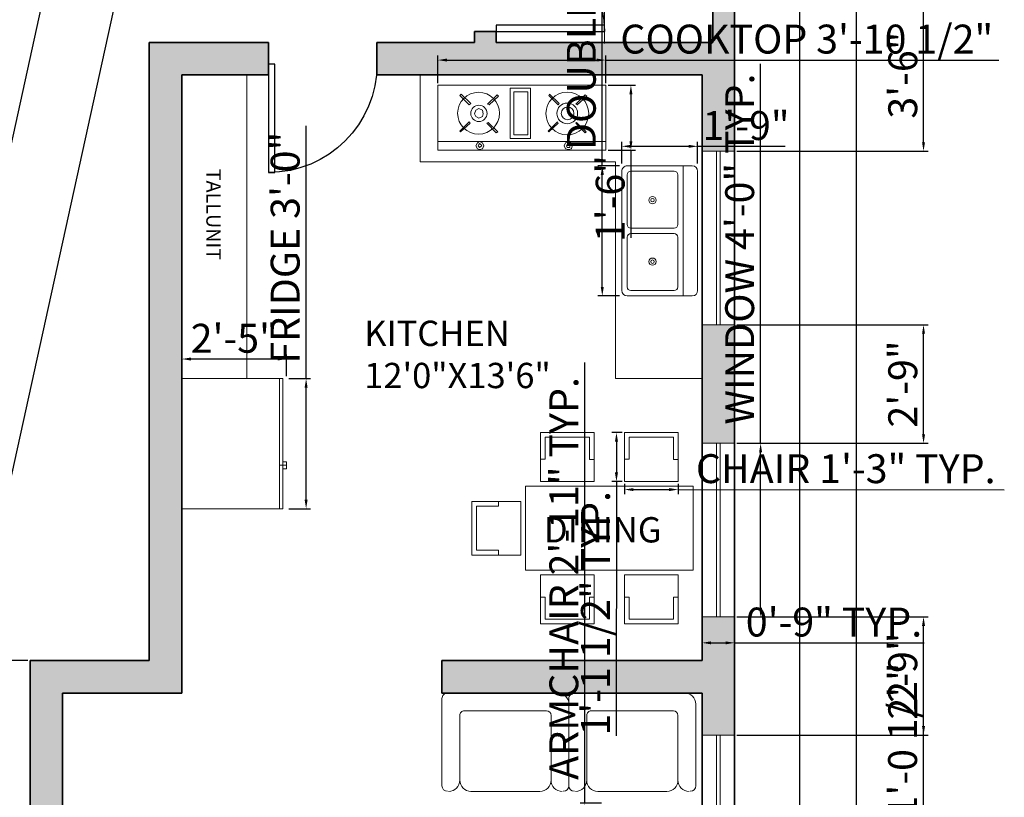
# Model space of a CAD drawing. Units: inches. Extents: x 2642 to 4124, y 1227 to 1973.
# Tile 5 of 7: x 3483 to 3756, y 1645 to 1860. Entities that reach past the tile are written whole.
import ezdxf

# ---------------------------------------------------------------- set-up
doc = ezdxf.new("R2010")
doc.units = ezdxf.units.IN
for name, color, linetype, lineweight in [('A-ANNO-DIMS', 2, 'Continuous', 18), ('A-ANNO-TEXT', 7, 'Continuous', 18), ('A-AREA-IDEN', 7, 'Continuous', 18), ('A-DOOR', 3, 'Continuous', 25), ('A-EQPM', 8, 'Continuous', 18), ('A-FLOR-CASE', 8, 'Continuous', 18), ('A-WALL', 7, 'Continuous', 35), ('A-WALL-PATT', 7, 'Continuous', 13), ('C-PROP', 7, 'Continuous', 25), ('furn', 165, 'Continuous', 18), ('window', 4, 'Continuous', 18), ('Сантехника', 9, 'Continuous', 18)]:
    doc.layers.add(name, color=color, linetype=linetype, lineweight=lineweight)
doc.styles.get("Standard").update_dxf_attribs({"font": 'arial.ttf'})
doc.dimstyles.new('ISO-25', dxfattribs={"dimtxt": 8, "dimasz": 2.5, "dimexe": 1.25, "dimexo": 0.625, "dimtad": 1, "dimdec": 0, "dimlunit": 3, "dimtxsty": 'Standard', "dimcen": 2.5, "dimadec": 0, "dimazin": 0, "dimtfac": 1, "dimtdec": 0, "dimtmove": 0, "dimatfit": 3, "dimfxl": 1, "dimarcsym": 0})

# ---------------------------------------------------------------- blocks, each defined once
blk = doc.blocks.new('*D2')
at = {"layer": 'A-ANNO-DIMS', "color": 0, "lineweight": -2, "transparency": 16777216}
for p, q in [((3699.85, 1907.78), (3716.14, 1907.78)), ((3714.89, 1905.28), (3714.89, 1310.28)), ((3699.85, 1307.78), (3716.14, 1307.78))]:
    blk.add_line(p, q, dxfattribs=at)
at = {"layer": 'A-ANNO-DIMS', "color": 0, "transparency": 16777216}
for points in [[(3714.47, 1905.28), (3715.3, 1905.28), (3714.89, 1907.78)], [(3714.47, 1310.28), (3715.3, 1310.28), (3714.89, 1307.78)]]:
    blk.add_solid(points, dxfattribs=at)
at = {"layer": 'Defpoints', "color": 0, "transparency": 16777216}
for p in [(3699.22, 1907.78), (3699.22, 1307.78), (3714.89, 1307.78)]:
    blk.add_point(p, dxfattribs=at)
at = {"layer": 'A-ANNO-DIMS', "color": 0, "transparency": 16777216, "insert": (3710.18, 1607.78), "char_height": 8, "attachment_point": 5, "rotation": 90}
blk.add_mtext("50'", dxfattribs=at)
blk = doc.blocks.new('*D4')
at = {"layer": 'A-ANNO-DIMS', "color": 0, "lineweight": -2, "transparency": 16777216}
for p, q in [((3518.61, 1907.92), (3498.8, 1912.28)), ((3368.56, 1314.45), (3499.49, 1909.57)), ((3386.61, 1307.92), (3366.8, 1312.28))]:
    blk.add_line(p, q, dxfattribs=at)
at = {"layer": 'A-ANNO-DIMS', "color": 0, "transparency": 16777216}
for points in [[(3499.08, 1909.65), (3499.89, 1909.48), (3500.02, 1912.01)], [(3368.15, 1314.54), (3368.97, 1314.36), (3368.02, 1312.01)]]:
    blk.add_solid(points, dxfattribs=at)
at = {"layer": 'Defpoints', "color": 0, "transparency": 16777216}
for p in [(3500.02, 1912.01), (3519.22, 1907.78), (3387.22, 1307.78)]:
    blk.add_point(p, dxfattribs=at)
at = {"layer": 'A-ANNO-DIMS', "color": 0, "transparency": 16777216, "insert": (3429.42, 1613.02), "char_height": 8, "attachment_point": 5, "rotation": 77.5926}
blk.add_mtext('51\'-2"', dxfattribs=at)
blk = doc.blocks.new('*U11')
for p, q in [((0, 0), (0, -6)), ((30, 0), (30, -6))]:
    blk.add_line(p, q)
blk.add_lwpolyline([(0, 0), (0, 30), (1.75, 30), (1.75, 0)], close=True)
blk.add_arc((0, 0), 30, 0, 90)
blk = doc.blocks.new('sofa-27')
at = {"color": 0, "linetype": 'ByBlock'}
for p, q in [((-0.0591, 0.0591), (-0.0591, 0.4902)), ((0.0945, 0.5198), (0.459, 0.5198)), ((0.6125, 0.0295), (0.6125, 0.4902)), ((0.0354, 0.1181), (0.0354, 0.4607)), ((0.518, 0.1181), (0.518, 0.4607)), ((0.4944, 0.0945), (0.0591, 0.0945)), ((0.583, 0), (0, 0))]:
    blk.add_line(p, q, dxfattribs=at)
for centre, radius, start, end in [((-0.0295, 0.4902), 0.0295, 90, 180), ((-0.0236, 0.4607), 0.0591, 360, 90), ((0.0945, 0.4607), 0.0591, 90, 180), ((0.459, 0.4607), 0.0591, 0, 90), ((0.5771, 0.4607), 0.0591, 90, 180), ((0.583, 0.4902), 0.0295, 0, 90), ((0.0591, 0.1181), 0.0236, 180, 270), ((0.4944, 0.1181), 0.0236, 270, 0), ((0, 0.0591), 0.0591, 180, 270), ((0.583, 0.0295), 0.0295, 270, 0)]:
    blk.add_arc(centre, radius, start, end, dxfattribs=at)
blk = doc.blocks.new('gas 1')
for points in [[(35.93, -1.87), (35.93, 0), (0, 0), (0, -1.87)], [(8.12, -0.94), (8.44, -1.56), (8.91, -1.87), (9.53, -1.56), (9.84, -0.94), (9.53, -0.31), (8.91, -0.16), (8.44, -0.31)], [(8.59, -0.94), (8.75, -1.25), (8.91, -1.41), (9.22, -1.25), (9.37, -0.94), (9.22, -0.78), (8.91, -0.62), (8.75, -0.78)], [(27.03, -0.94), (27.34, -1.56), (27.97, -1.87), (28.59, -1.56), (28.75, -0.94), (28.59, -0.31), (27.97, -0.16), (27.34, -0.31)], [(27.5, -0.94), (27.65, -1.25), (27.97, -1.41), (28.28, -1.25), (28.28, -0.94), (28.28, -0.62), (27.97, -0.62), (27.65, -0.62)], [(4.84, -3.91), (4.69, -4.06), (6.72, -6.09), (6.87, -5.78)], [(12.81, -3.91), (12.5, -3.75), (10.47, -5.78), (10.78, -5.94)], [(19.84, -13.28), (15.47, -13.28), (15.47, -2.5), (19.84, -2.5)], [(19.22, -12.5), (16.25, -12.5), (16.25, -3.28), (19.22, -3.28)], [(23.75, -3.91), (23.59, -4.06), (25.62, -6.09), (25.78, -5.78)], [(31.71, -3.91), (31.56, -3.75), (29.53, -5.78), (29.68, -5.94)], [(7.81, -7.81), (8.12, -8.59), (8.75, -8.91), (9.53, -8.59), (9.69, -7.81), (9.53, -7.19), (8.75, -6.87), (8.12, -7.19)], [(7.03, -10), (6.72, -9.69), (4.69, -11.72), (5, -12.03)], [(12.97, -11.56), (10.94, -9.69), (10.62, -9.84), (12.65, -11.87)], [(23.75, -11.72), (23.9, -12.03), (25.93, -10), (25.78, -9.69)], [(31.87, -11.56), (29.84, -9.69), (29.53, -9.84), (31.56, -11.87)]]:
    blk.add_lwpolyline(points, close=True)
blk.add_lwpolyline([(35.93, -1.87), (35.93, -13.9), (0, -13.9), (0, -1.87)])
for centre, radius in [((8.7, -7.92), 4.48), ((27.7, -7.86), 4.58), ((8.77, -7.89), 1.74), ((27.69, -7.89), 2.22), ((27.76, -7.89), 1.35)]:
    blk.add_circle(centre, radius)
blk = doc.blocks.new('Sink-double - 36 in top')
for p, q in [((-18, -4), (18, -4)), ((-0.75, -18.5), (-0.75, -6.5)), ((0.75, -6.5), (0.75, -18.5))]:
    blk.add_line(p, q)
for points in [[(-16.5, 0), (16.5, 0)], [(-18, -19.5), (-18, -1.5)], [(18, -1.5), (18, -19.5)], [(-16.5, -18.5), (-16.5, -6.5)], [(-15.5, -5.5), (-1.75, -5.5)], [(1.75, -5.5), (15.5, -5.5)], [(16.5, -6.5), (16.5, -18.5)], [(16.5, -21), (-16.5, -21)], [(-1.75, -19.5), (-15.5, -19.5)], [(15.5, -19.5), (1.75, -19.5)]]:
    blk.add_lwpolyline(points)
for centre, radius in [((-8.5, -12.5), 1), ((-8.5, -12.5), 0.5), ((8.5, -12.5), 1), ((8.5, -12.5), 0.5)]:
    blk.add_circle(centre, radius)
for centre, radius, start, end in [((-16.5, -1.5), 1.5, 90, 180), ((16.5, -1.5), 1.5, 0, 90), ((-15.5, -6.5), 1, 90, 180), ((-1.75, -6.5), 1, 0, 90), ((1.75, -6.5), 1, 90, 180), ((15.5, -6.5), 1, 0, 90), ((-15.5, -18.5), 1, 180, 270), ((-1.75, -18.5), 1, 270, 0), ((1.75, -18.5), 1, 180, 270), ((15.5, -18.5), 1, 270, 0), ((-16.5, -19.5), 1.5, 180, 270), ((16.5, -19.5), 1.5, 270, 0)]:
    blk.add_arc(centre, radius, start, end)
blk = doc.blocks.new('Refrigerator-2 door - 36 in top')
for p, q in [((0, -26.999999), (36, -26.999999)), ((12, -26.999999), (12, -28.999999)), ((11, -27.999999), (11, -28.999999)), ((11, -28.999999), (13, -28.999999)), ((13, -28.999999), (13, -27.999999))]:
    blk.add_line(p, q)
blk.add_lwpolyline([(0, -27.999999), (0, 0), (36, 0), (36, -27.999999)], close=True)
blk = doc.blocks.new('CHAIR-DINING')
for p, q in [((0, 14.84), (13.57, 14.84)), ((0, 0), (0, 14.84)), ((7.42, 13.56), (7.42, 14.84)), ((13.57, 0), (13.57, 14.84)), ((1.28, 13.56), (7.42, 13.56)), ((1.28, 1.32), (1.28, 13.56)), ((0, 0), (13.57, 0)), ((7.42, 1.32), (1.28, 1.32)), ((7.42, 0), (7.42, 1.32))]:
    blk.add_line(p, q)
blk = doc.blocks.new('WIN-24IN')
for p, q in [((0, 24), (9, 24)), ((4, 24), (4, 0)), ((5, 24), (5, 0)), ((0, 0), (9, 0))]:
    blk.add_line(p, q)
blk = doc.blocks.new('WIN-48IN')
for p, q in [((9, 48), (0, 48)), ((4, 48), (4, 0)), ((5, 48), (5, 0)), ((9, 0), (0, 0))]:
    blk.add_line(p, q)
blk = doc.blocks.new('*D38')
at = {"layer": 'A-ANNO-DIMS', "color": 0, "lineweight": -2, "transparency": 16777216}
for p, q in [((3650.74, 1731.67), (3650.74, 1728.82)), ((3665.58, 1731.67), (3665.58, 1728.82)), ((3653.24, 1730.07), (3663.08, 1730.07)), ((3665.58, 1730.07), (3755.88, 1730.03))]:
    blk.add_line(p, q, dxfattribs=at)
at = {"layer": 'A-ANNO-DIMS', "color": 0, "transparency": 16777216}
for points in [[(3653.24, 1730.49), (3653.24, 1729.65), (3650.74, 1730.07)], [(3663.08, 1730.48), (3663.08, 1729.65), (3665.58, 1730.07)]]:
    blk.add_solid(points, dxfattribs=at)
at = {"layer": 'Defpoints', "color": 0, "transparency": 16777216}
for p in [(3650.74, 1732.3), (3665.58, 1732.29), (3665.58, 1730.07)]:
    blk.add_point(p, dxfattribs=at)
at = {"layer": 'A-ANNO-DIMS', "color": 0, "transparency": 16777216, "insert": (3711.98, 1734.81), "char_height": 8, "attachment_point": 5, "rotation": 359.979}
blk.add_mtext('CHAIR 1\'-3" TYP.', dxfattribs=at)
blk = doc.blocks.new('*D39')
at = {"layer": 'A-ANNO-DIMS', "color": 0, "lineweight": -2, "transparency": 16777216}
for p, q in [((3650.12, 1745.86), (3647.27, 1745.87)), ((3648.52, 1743.36), (3648.52, 1734.8)), ((3650.12, 1732.3), (3647.27, 1732.3)), ((3648.52, 1732.3), (3648.49, 1661.9))]:
    blk.add_line(p, q, dxfattribs=at)
at = {"layer": 'A-ANNO-DIMS', "color": 0, "transparency": 16777216}
for points in [[(3648.11, 1743.37), (3648.94, 1743.36), (3648.52, 1745.86)], [(3648.1, 1734.8), (3648.94, 1734.8), (3648.52, 1732.3)]]:
    blk.add_solid(points, dxfattribs=at)
at = {"layer": 'Defpoints', "color": 0, "transparency": 16777216}
for p in [(3650.75, 1745.86), (3648.52, 1732.3), (3650.74, 1732.3)]:
    blk.add_point(p, dxfattribs=at)
at = {"layer": 'A-ANNO-DIMS', "color": 0, "transparency": 16777216, "insert": (3643.74, 1695.85), "char_height": 8, "attachment_point": 5, "rotation": 89.979}
blk.add_mtext('1\'-1 1/2" TYP.', dxfattribs=at)
blk = doc.blocks.new('*D40')
at = {"layer": 'A-ANNO-DIMS', "color": 0, "lineweight": -2, "transparency": 16777216}
for p, q in [((3639.76, 1643.28), (3639.76, 1765.19)), ((3644.41, 1643.28), (3638.51, 1643.28)), ((3639.76, 1610.65), (3639.76, 1640.78)), ((3644.41, 1608.15), (3638.51, 1608.15))]:
    blk.add_line(p, q, dxfattribs=at)
at = {"layer": 'A-ANNO-DIMS', "color": 0, "transparency": 16777216}
for points in [[(3639.34, 1640.78), (3640.18, 1640.78), (3639.76, 1643.28)], [(3639.34, 1610.65), (3640.18, 1610.65), (3639.76, 1608.15)]]:
    blk.add_solid(points, dxfattribs=at)
at = {"layer": 'Defpoints', "color": 0, "transparency": 16777216}
for p in [(3639.76, 1643.28), (3645.03, 1643.28), (3645.03, 1608.15)]:
    blk.add_point(p, dxfattribs=at)
at = {"layer": 'A-ANNO-DIMS', "color": 0, "transparency": 16777216, "insert": (3635, 1705.48), "char_height": 8, "attachment_point": 5, "rotation": 90}
blk.add_mtext('ARMCHAIR 2\'-11" TYP.', dxfattribs=at)
blk = doc.blocks.new('*D44')
at = {"layer": 'A-ANNO-DIMS', "color": 0, "lineweight": -2, "transparency": 16777216}
for p, q in [((3688.42, 1742.87), (3688.42, 1847.85)), ((3681.85, 1742.87), (3689.67, 1742.87)), ((3688.42, 1697.37), (3688.42, 1740.37)), ((3681.85, 1694.87), (3689.67, 1694.87))]:
    blk.add_line(p, q, dxfattribs=at)
at = {"layer": 'A-ANNO-DIMS', "color": 0, "transparency": 16777216}
for points in [[(3688.01, 1740.37), (3688.84, 1740.37), (3688.42, 1742.87)], [(3688.01, 1697.37), (3688.84, 1697.37), (3688.42, 1694.87)]]:
    blk.add_solid(points, dxfattribs=at)
at = {"layer": 'Defpoints', "color": 0, "transparency": 16777216}
for p in [(3681.22, 1742.87), (3688.42, 1742.87), (3681.22, 1694.87)]:
    blk.add_point(p, dxfattribs=at)
at = {"layer": 'A-ANNO-DIMS', "color": 0, "transparency": 16777216, "insert": (3683.66, 1796.61), "char_height": 8, "attachment_point": 5, "rotation": 90}
blk.add_mtext('WINDOW 4\'-0" TYP.', dxfattribs=at)
blk = doc.blocks.new('*D45')
at = {"layer": 'A-ANNO-DIMS', "color": 0, "lineweight": -2, "transparency": 16777216}
for p, q in [((3672.22, 1694.24), (3672.22, 1686.42)), ((3681.22, 1694.24), (3681.22, 1686.42)), ((3674.72, 1687.67), (3678.72, 1687.67)), ((3681.22, 1687.67), (3733.74, 1687.67))]:
    blk.add_line(p, q, dxfattribs=at)
at = {"layer": 'A-ANNO-DIMS', "color": 0, "transparency": 16777216}
for points in [[(3674.72, 1688.08), (3674.72, 1687.25), (3672.22, 1687.67)], [(3678.72, 1688.08), (3678.72, 1687.25), (3681.22, 1687.67)]]:
    blk.add_solid(points, dxfattribs=at)
at = {"layer": 'Defpoints', "color": 0, "transparency": 16777216}
for p in [(3672.22, 1694.87), (3681.22, 1694.87), (3681.22, 1687.67)]:
    blk.add_point(p, dxfattribs=at)
at = {"layer": 'A-ANNO-DIMS', "color": 0, "transparency": 16777216, "insert": (3708.73, 1692.38), "char_height": 8, "attachment_point": 5}
blk.add_mtext('0\'-9" TYP.', dxfattribs=at)
blk = doc.blocks.new('*D58')
at = {"layer": 'A-ANNO-DIMS', "color": 0, "lineweight": -2, "transparency": 16777216}
for p, q in [((3599.11, 1842.55), (3599.11, 1850.14)), ((3601.61, 1848.89), (3643.06, 1848.89)), ((3645.56, 1842.55), (3645.56, 1850.14)), ((3645.56, 1848.89), (3754.33, 1848.89))]:
    blk.add_line(p, q, dxfattribs=at)
at = {"layer": 'A-ANNO-DIMS', "color": 0, "transparency": 16777216}
for points in [[(3601.61, 1849.31), (3601.61, 1848.48), (3599.11, 1848.89)], [(3643.06, 1849.31), (3643.06, 1848.48), (3645.56, 1848.89)]]:
    blk.add_solid(points, dxfattribs=at)
at = {"layer": 'Defpoints', "color": 0, "transparency": 16777216}
for p in [(3645.56, 1848.89), (3599.11, 1841.93), (3645.56, 1841.93)]:
    blk.add_point(p, dxfattribs=at)
at = {"layer": 'A-ANNO-DIMS', "color": 0, "transparency": 16777216, "insert": (3701.2, 1853.66), "char_height": 8, "attachment_point": 5}
blk.add_mtext('COOKTOP 3\'-10 1/2"', dxfattribs=at)
blk = doc.blocks.new('*D59')
at = {"layer": 'A-ANNO-DIMS', "color": 0, "lineweight": -2, "transparency": 16777216}
for p, q in [((3646.19, 1841.93), (3653.78, 1841.93)), ((3652.53, 1839.43), (3652.53, 1826.45)), ((3646.19, 1823.95), (3653.78, 1823.95)), ((3652.53, 1823.95), (3652.53, 1799.69))]:
    blk.add_line(p, q, dxfattribs=at)
at = {"layer": 'A-ANNO-DIMS', "color": 0, "transparency": 16777216}
for points in [[(3652.11, 1839.43), (3652.94, 1839.43), (3652.53, 1841.93)], [(3652.11, 1826.45), (3652.94, 1826.45), (3652.53, 1823.95)]]:
    blk.add_solid(points, dxfattribs=at)
at = {"layer": 'Defpoints', "color": 0, "transparency": 16777216}
for p in [(3645.56, 1841.93), (3645.56, 1823.95), (3652.53, 1823.95)]:
    blk.add_point(p, dxfattribs=at)
at = {"layer": 'A-ANNO-DIMS', "color": 0, "transparency": 16777216, "insert": (3647.82, 1810.57), "char_height": 8, "attachment_point": 5, "rotation": 90}
blk.add_mtext('1\'-6"', dxfattribs=at)
blk = doc.blocks.new('*D60')
at = {"layer": 'A-ANNO-DIMS', "color": 0, "lineweight": -2, "transparency": 16777216}
for p, q in [((3644.6, 1819.63), (3644.6, 1922.5)), ((3649.37, 1819.63), (3643.35, 1819.63)), ((3644.6, 1786.13), (3644.6, 1817.13)), ((3649.37, 1783.63), (3643.35, 1783.63))]:
    blk.add_line(p, q, dxfattribs=at)
at = {"layer": 'A-ANNO-DIMS', "color": 0, "transparency": 16777216}
for points in [[(3644.18, 1817.13), (3645.02, 1817.13), (3644.6, 1819.63)], [(3644.18, 1786.13), (3645.02, 1786.13), (3644.6, 1783.63)]]:
    blk.add_solid(points, dxfattribs=at)
at = {"layer": 'Defpoints', "color": 0, "transparency": 16777216}
for p in [(3644.6, 1819.63), (3650, 1819.63), (3650, 1783.63)]:
    blk.add_point(p, dxfattribs=at)
at = {"layer": 'A-ANNO-DIMS', "color": 0, "transparency": 16777216, "insert": (3639.83, 1872.32), "char_height": 8, "attachment_point": 5, "rotation": 90}
blk.add_mtext('DOUBLE SINK 3\'-0"', dxfattribs=at)
blk = doc.blocks.new('*D61')
at = {"layer": 'A-ANNO-DIMS', "color": 0, "lineweight": -2, "transparency": 16777216}
for p, q in [((3650, 1820.26), (3650, 1826.28)), ((3671, 1820.26), (3671, 1826.28)), ((3652.5, 1825.03), (3668.5, 1825.03)), ((3671, 1825.03), (3695.26, 1825.03))]:
    blk.add_line(p, q, dxfattribs=at)
at = {"layer": 'A-ANNO-DIMS', "color": 0, "transparency": 16777216}
for points in [[(3652.5, 1825.45), (3652.5, 1824.62), (3650, 1825.03)], [(3668.5, 1825.45), (3668.5, 1824.62), (3671, 1825.03)]]:
    blk.add_solid(points, dxfattribs=at)
at = {"layer": 'Defpoints', "color": 0, "transparency": 16777216}
for p in [(3671, 1825.03), (3650, 1819.63), (3671, 1819.63)]:
    blk.add_point(p, dxfattribs=at)
at = {"layer": 'A-ANNO-DIMS', "color": 0, "transparency": 16777216, "insert": (3684.38, 1829.74), "char_height": 8, "attachment_point": 5}
blk.add_mtext('1\'-9"', dxfattribs=at)
blk = doc.blocks.new('*D66')
at = {"layer": 'A-ANNO-DIMS', "color": 0, "lineweight": -2, "transparency": 16777216}
for p, q in [((3562.62, 1760.78), (3562.62, 1830.67)), ((3557.85, 1760.78), (3563.87, 1760.78)), ((3562.62, 1727.28), (3562.62, 1758.28)), ((3557.85, 1724.78), (3563.87, 1724.78))]:
    blk.add_line(p, q, dxfattribs=at)
at = {"layer": 'A-ANNO-DIMS', "color": 0, "transparency": 16777216}
for points in [[(3562.21, 1758.28), (3563.04, 1758.28), (3562.62, 1760.78)], [(3562.21, 1727.28), (3563.04, 1727.28), (3562.62, 1724.78)]]:
    blk.add_solid(points, dxfattribs=at)
at = {"layer": 'Defpoints', "color": 0, "transparency": 16777216}
for p in [(3557.22, 1760.78), (3562.62, 1760.78), (3557.22, 1724.78)]:
    blk.add_point(p, dxfattribs=at)
at = {"layer": 'A-ANNO-DIMS', "color": 0, "transparency": 16777216, "insert": (3557.86, 1796.98), "char_height": 8, "attachment_point": 5, "rotation": 90}
blk.add_mtext('FRIDGE 3\'-0"', dxfattribs=at)
blk = doc.blocks.new('*D67')
at = {"layer": 'A-ANNO-DIMS', "color": 0, "lineweight": -2, "transparency": 16777216}
for p, q in [((3528.22, 1761.41), (3528.22, 1767.43)), ((3554.72, 1766.18), (3530.72, 1766.18)), ((3557.22, 1761.41), (3557.22, 1767.43))]:
    blk.add_line(p, q, dxfattribs=at)
at = {"layer": 'A-ANNO-DIMS', "color": 0, "transparency": 16777216}
for points in [[(3530.72, 1766.6), (3530.72, 1765.77), (3528.22, 1766.18)], [(3554.72, 1766.6), (3554.72, 1765.77), (3557.22, 1766.18)]]:
    blk.add_solid(points, dxfattribs=at)
at = {"layer": 'Defpoints', "color": 0, "transparency": 16777216}
for p in [(3528.22, 1766.18), (3528.22, 1760.78), (3557.22, 1760.78)]:
    blk.add_point(p, dxfattribs=at)
at = {"layer": 'A-ANNO-DIMS', "color": 0, "transparency": 16777216, "insert": (3542.72, 1770.89), "char_height": 8, "attachment_point": 5}
blk.add_mtext('2\'-5"', dxfattribs=at)
blk = doc.blocks.new('*D70')
at = {"layer": 'A-ANNO-DIMS', "color": 0, "lineweight": -2, "transparency": 16777216}
for p, q in [((3518.6, 1907.78), (3351.67, 1907.78)), ((3352.92, 1905.28), (3352.92, 1685.28)), ((3485.6, 1682.78), (3351.67, 1682.78))]:
    blk.add_line(p, q, dxfattribs=at)
at = {"layer": 'A-ANNO-DIMS', "color": 0, "transparency": 16777216}
for points in [[(3352.51, 1905.28), (3353.34, 1905.28), (3352.92, 1907.78)], [(3352.51, 1685.28), (3353.34, 1685.28), (3352.92, 1682.78)]]:
    blk.add_solid(points, dxfattribs=at)
at = {"layer": 'Defpoints', "color": 0, "transparency": 16777216}
for p in [(3519.22, 1907.78), (3352.92, 1682.78), (3486.22, 1682.78)]:
    blk.add_point(p, dxfattribs=at)
at = {"layer": 'A-ANNO-DIMS', "color": 0, "transparency": 16777216, "insert": (3348.21, 1795.28), "char_height": 8, "attachment_point": 5, "rotation": 90}
blk.add_mtext('18\'-9"', dxfattribs=at)
blk = doc.blocks.new('*D78')
at = {"layer": 'A-ANNO-DIMS', "color": 0, "lineweight": -2, "transparency": 16777216}
for p, q in [((3733.52, 1638.12), (3733.52, 1681.02)), ((3681.85, 1638.12), (3734.77, 1638.12)), ((3733.52, 1628.28), (3733.52, 1635.62)), ((3681.85, 1625.78), (3734.77, 1625.78))]:
    blk.add_line(p, q, dxfattribs=at)
at = {"layer": 'A-ANNO-DIMS', "color": 0, "transparency": 16777216}
for points in [[(3733.11, 1635.62), (3733.94, 1635.62), (3733.52, 1638.12)], [(3733.11, 1628.28), (3733.94, 1628.28), (3733.52, 1625.78)]]:
    blk.add_solid(points, dxfattribs=at)
at = {"layer": 'Defpoints', "color": 0, "transparency": 16777216}
for p in [(3681.22, 1638.12), (3733.52, 1638.12), (3681.22, 1625.78)]:
    blk.add_point(p, dxfattribs=at)
at = {"layer": 'A-ANNO-DIMS', "color": 0, "transparency": 16777216, "insert": (3728.76, 1660.82), "char_height": 8, "attachment_point": 5, "rotation": 90}
blk.add_mtext('1\'-0 1/2"', dxfattribs=at)
blk = doc.blocks.new('*D79')
at = {"layer": 'A-ANNO-DIMS', "color": 0, "lineweight": -2, "transparency": 16777216}
for p, q in [((3681.85, 1694.87), (3734.77, 1694.87)), ((3733.52, 1664.62), (3733.52, 1692.37)), ((3681.85, 1662.12), (3734.77, 1662.12))]:
    blk.add_line(p, q, dxfattribs=at)
at = {"layer": 'A-ANNO-DIMS', "color": 0, "transparency": 16777216}
for points in [[(3733.11, 1692.37), (3733.94, 1692.37), (3733.52, 1694.87)], [(3733.11, 1664.62), (3733.94, 1664.62), (3733.52, 1662.12)]]:
    blk.add_solid(points, dxfattribs=at)
at = {"layer": 'Defpoints', "color": 0, "transparency": 16777216}
for p in [(3681.22, 1694.87), (3733.52, 1694.87), (3681.22, 1662.12)]:
    blk.add_point(p, dxfattribs=at)
at = {"layer": 'A-ANNO-DIMS', "color": 0, "transparency": 16777216, "insert": (3728.81, 1678.49), "char_height": 8, "attachment_point": 5, "rotation": 90}
blk.add_mtext('2\'-9"', dxfattribs=at)
blk = doc.blocks.new('*D80')
at = {"layer": 'A-ANNO-DIMS', "color": 0, "lineweight": -2, "transparency": 16777216}
for p, q in [((3681.85, 1775.67), (3734.77, 1775.67)), ((3733.52, 1745.37), (3733.52, 1773.17)), ((3681.85, 1742.87), (3734.77, 1742.87))]:
    blk.add_line(p, q, dxfattribs=at)
at = {"layer": 'A-ANNO-DIMS', "color": 0, "transparency": 16777216}
for points in [[(3733.11, 1773.17), (3733.94, 1773.17), (3733.52, 1775.67)], [(3733.11, 1745.37), (3733.94, 1745.37), (3733.52, 1742.87)]]:
    blk.add_solid(points, dxfattribs=at)
at = {"layer": 'Defpoints', "color": 0, "transparency": 16777216}
for p in [(3681.22, 1775.67), (3733.52, 1775.67), (3681.22, 1742.87)]:
    blk.add_point(p, dxfattribs=at)
at = {"layer": 'A-ANNO-DIMS', "color": 0, "transparency": 16777216, "insert": (3728.81, 1759.27), "char_height": 8, "attachment_point": 5, "rotation": 90}
blk.add_mtext('2\'-9"', dxfattribs=at)
blk = doc.blocks.new('*D81')
at = {"layer": 'A-ANNO-DIMS', "color": 0, "lineweight": -2, "transparency": 16777216}
for p, q in [((3681.85, 1865.78), (3734.77, 1865.78)), ((3733.52, 1826.17), (3733.52, 1863.28)), ((3681.85, 1823.67), (3734.77, 1823.67))]:
    blk.add_line(p, q, dxfattribs=at)
at = {"layer": 'A-ANNO-DIMS', "color": 0, "transparency": 16777216}
for points in [[(3733.11, 1863.28), (3733.94, 1863.28), (3733.52, 1865.78)], [(3733.11, 1826.17), (3733.94, 1826.17), (3733.52, 1823.67)]]:
    blk.add_solid(points, dxfattribs=at)
at = {"layer": 'Defpoints', "color": 0, "transparency": 16777216}
for p in [(3681.22, 1865.78), (3733.52, 1865.78), (3681.22, 1823.67)]:
    blk.add_point(p, dxfattribs=at)
at = {"layer": 'A-ANNO-DIMS', "color": 0, "transparency": 16777216, "insert": (3728.81, 1844.73), "char_height": 8, "attachment_point": 5, "rotation": 90}
blk.add_mtext('3\'-6"', dxfattribs=at)

msp = doc.modelspace()

# ---------------------------------------------------------------- hatches: boundary and pattern name
at = {"layer": 'A-WALL-PATT'}
h = msp.add_hatch(color=256, dxfattribs=at)
h.dxf.hatch_style = 1
h.paths.add_polyline_path([(3552.22, 1505.78), (3495.22, 1505.78), (3495.22, 1508.78), (3492.22, 1508.78), (3486.22, 1508.78), (3486.22, 1415.78), (3495.22, 1415.78), (3495.22, 1499.78), (3543.22, 1499.78), (3543.22, 1457.78), (3549.22, 1457.78), (3549.22, 1499.78), (3552.19, 1499.78), (3552.19, 1499.78)])
h.paths.add_polyline_path([(3681.22, 1427.78), (3672.22, 1427.78), (3672.22, 1395.07), (3672.22, 1379.78), (3549.22, 1379.78), (3549.22, 1427.78), (3543.22, 1427.78), (3543.22, 1379.78), (3495.22, 1379.78), (3495.22, 1391.78), (3486.22, 1391.78), (3486.22, 1370.78), (3675.22, 1370.78), (3675.22, 1307.78), (3681.22, 1307.78)])
h.paths.add_polyline_path([(3681.22, 1517.78), (3672.22, 1517.78), (3672.22, 1505.78), (3640.73, 1505.78), (3588.22, 1505.78), (3588.22, 1499.78), (3672.22, 1499.78), (3672.22, 1475.78), (3681.22, 1475.78)])
h.paths.add_polyline_path([(3681.22, 1638.12), (3672.22, 1638.12), (3672.22, 1625.78), (3681.22, 1625.78)])
h.paths.add_polyline_path([(3681.22, 1553.78), (3672.22, 1553.78), (3672.22, 1541.78), (3681.22, 1541.78)])
h.paths.add_polyline_path([(3528.22, 1844.78), (3552.22, 1844.78), (3552.22, 1847.78), (3552.22, 1853.78), (3519.22, 1853.78), (3519.22, 1682.78), (3486.22, 1682.78), (3486.22, 1548.78), (3492.22, 1548.78), (3495.22, 1548.78), (3495.22, 1673.78), (3528.22, 1673.78)])
h.paths.add_polyline_path([(3681.22, 1865.78), (3675.22, 1865.78), (3675.22, 1853.78), (3615.22, 1853.78), (3615.22, 1856.78), (3609.22, 1856.78), (3609.22, 1853.78), (3582.22, 1853.78), (3582.22, 1847.78), (3582.22, 1844.78), (3672.22, 1844.78), (3672.22, 1823.67), (3681.22, 1823.67)])
h.paths.add_polyline_path([(3681.22, 1907.78), (3519.22, 1907.78), (3519.22, 1901.78), (3540.68, 1901.78), (3609.22, 1901.78), (3609.22, 1886.78), (3615.22, 1886.78), (3615.22, 1901.78), (3675.22, 1901.78), (3675.22, 1889.78), (3681.22, 1889.78)])
h.paths.add_polyline_path([(3681.22, 1775.67), (3672.22, 1775.67), (3672.22, 1742.87), (3681.22, 1742.87)])
h.paths.add_polyline_path([(3681.22, 1694.87), (3672.22, 1694.87), (3672.22, 1682.78), (3600.22, 1682.78), (3600.22, 1673.78), (3672.22, 1673.78), (3672.22, 1662.12), (3681.22, 1662.12)])

# ---------------------------------------------------------------- linework, layer by layer
at = {"layer": 'A-FLOR-CASE'}
for p, q in [((3546.22, 1844.78), (3546.22, 1760.78)), ((3594.22, 1844.78), (3594.22, 1820.78)), ((3648.22, 1820.78), (3594.22, 1820.78)), ((3648.22, 1820.78), (3648.22, 1760.78)), ((3546.22, 1760.78), (3528.22, 1760.78)), ((3672.22, 1760.78), (3648.22, 1760.78))]:
    msp.add_line(p, q, dxfattribs=at)
at = {"layer": 'A-WALL'}
for p, q in [((3681.22, 1907.78), (3681.22, 1307.78)), ((3675.22, 1901.78), (3675.22, 1853.78)), ((3615.22, 1856.78), (3609.22, 1856.78)), ((3609.22, 1856.78), (3609.22, 1853.78)), ((3615.22, 1856.78), (3615.22, 1853.78)), ((3519.22, 1853.78), (3519.22, 1682.78)), ((3552.22, 1853.78), (3519.22, 1853.78)), ((3552.22, 1853.78), (3552.22, 1844.78)), ((3609.22, 1853.78), (3582.22, 1853.78)), ((3582.22, 1853.78), (3582.22, 1844.78)), ((3675.22, 1853.78), (3615.22, 1853.78)), ((3528.22, 1844.78), (3528.22, 1673.78)), ((3552.22, 1844.78), (3528.22, 1844.78)), ((3672.22, 1844.78), (3582.22, 1844.78)), ((3672.22, 1844.78), (3672.22, 1682.78)), ((3486.22, 1682.78), (3486.22, 1548.78)), ((3519.22, 1682.78), (3486.22, 1682.78)), ((3672.22, 1682.78), (3600.22, 1682.78)), ((3600.22, 1682.78), (3600.22, 1673.78)), ((3495.22, 1673.78), (3495.22, 1548.78)), ((3528.22, 1673.78), (3495.22, 1673.78)), ((3672.22, 1673.78), (3600.22, 1673.78)), ((3672.22, 1673.78), (3672.22, 1505.78))]:
    msp.add_line(p, q, dxfattribs=at)
at = {"layer": 'C-PROP'}
for p, q in [((3519.22, 1907.78), (3387.22, 1307.78)), ((3699.22, 1907.78), (3699.22, 1307.78))]:
    msp.add_line(p, q, dxfattribs=at)
at = {"layer": 'furn'}
for p, q in [((3623.31, 1731.03), (3669.79, 1731.03)), ((3623.31, 1707.77), (3623.31, 1731.03)), ((3669.79, 1731.03), (3669.79, 1707.77)), ((3669.79, 1707.77), (3623.31, 1707.77))]:
    msp.add_line(p, q, dxfattribs=at)
at = {"layer": 'Сантехника'}
msp.add_line((3645.21, 1901.48), (3645.21, 1853.48), dxfattribs=at)

# ---------------------------------------------------------------- block references
at = {"layer": 'A-DOOR', "xscale": -1}
for p, rotation in [((3615.22, 1856.78), 270), ((3552.22, 1847.78), 180)]:
    msp.add_blockref('*U11', p, dxfattribs=dict(at, rotation=rotation))
at = {"layer": 'A-EQPM', "xscale": -1.292580420916565, "yscale": 1.292580420916565, "zscale": 1.292580420916565, "rotation": 180}
msp.add_blockref('gas 1', (3599.11, 1823.95), dxfattribs=at)
at = {"layer": 'A-EQPM', "rotation": 90}
msp.add_blockref('Refrigerator-2 door - 36 in top', (3528.22, 1724.78), dxfattribs=at)
at = {"layer": 'furn'}
for p, rotation in [((3627.5, 1745.87), 269.9293303373268), ((3650.75, 1745.86), 269.9790238270793), ((3642.36, 1692.93), 90.03023468099668), ((3665.6, 1692.93), 90.01148952387457)]:
    msp.add_blockref('CHAIR-DINING', p, dxfattribs=dict(at, rotation=rotation))
msp.add_blockref('CHAIR-DINING', (3608.46, 1711.96), dxfattribs=at)
at = {"layer": 'furn', "xscale": 52.31545737226423, "yscale": 52.31545737226423, "zscale": 52.31545737226423, "rotation": 180}
for p in [(3632.27, 1673.78), (3667.4, 1673.78)]:
    msp.add_blockref('sofa-27', p, dxfattribs=at)
at = {"layer": 'window'}
for name, p in [('WIN-48IN', (3672.22, 1775.67)), ('WIN-48IN', (3672.22, 1694.87)), ('WIN-24IN', (3672.22, 1638.12))]:
    msp.add_blockref(name, p, dxfattribs=at)
at = {"layer": 'Сантехника', "xscale": -1, "rotation": 270}
msp.add_blockref('Sink-double - 36 in top', (3671, 1801.63), dxfattribs=at)

# ---------------------------------------------------------------- texts
at = {"layer": 'A-ANNO-TEXT', "insert": (3539.01, 1818.83), "char_height": 4, "attachment_point": 1, "rotation": 270}
msp.add_mtext_dynamic_manual_height_columns('TALLUNIT', width=4, gutter_width=12.5, heights=[0], dxfattribs=at)
at = {"layer": 'A-AREA-IDEN', "char_height": 7, "attachment_point": 1}
for s, insert in [('{\\fTimes New Roman|b0|i0|c0|p18;KITCHEN\\P12\'0"X13\'6"}', (3578.71, 1776.8)), ('{\\fTimes New Roman|b0|i0|c0|p18;DINING}', (3628.46, 1722.44))]:
    msp.add_mtext_dynamic_manual_height_columns(s, width=61.0557, gutter_width=12.5, heights=[0], dxfattribs=dict(at, insert=insert))

# ---------------------------------------------------------------- dimensions: what is measured, and where the dimension line sits
at = {"layer": 'A-ANNO-DIMS'}
for base, p1, p2, angle, text, picture, middle in [((3644.6, 1819.63), (3650, 1783.63), (3650, 1819.63), 90, 'DOUBLE SINK <>', '*D60', (3639.83, 1872.32)), ((3688.42, 1742.87), (3681.22, 1694.87), (3681.22, 1742.87), 90, 'WINDOW <> TYP.', '*D44', (3683.66, 1796.61)), ((3562.62, 1760.78), (3557.22, 1724.78), (3557.22, 1760.78), 90, 'FRIDGE <>', '*D66', (3557.86, 1796.98)), ((3639.76, 1643.28), (3645.03, 1608.15), (3645.03, 1643.28), 90, 'ARMCHAIR <> TYP.', '*D40', (3635, 1705.48)), ((3665.58, 1730.07), (3650.74, 1732.3), (3665.58, 1732.29), 359.979, 'CHAIR <> TYP.', '*D38', (3711.98, 1734.81)), ((3648.52, 1732.3), (3650.75, 1745.86), (3650.74, 1732.3), 269.979, '<> TYP.', '*D39', (3643.74, 1695.85))]:
    dim = msp.add_linear_dim(base=base, p1=p1, p2=p2, angle=angle, text=text, dimstyle='ISO-25', override={"dimdec": 1, "dimlfac": 1, "dimrnd": 0, "dimzin": 1, "dimdsep": 46, "dimlunit": 4, "dimfrac": 2}, dxfattribs=at)
    dim.commit()
    dim.dimension.update_dxf_attribs({"geometry": picture, "text_midpoint": middle})
dim = msp.add_aligned_dim(p1=(3387.22, 1307.78), p2=(3519.22, 1907.78), distance=19.66, dimstyle='ISO-25', override={"dimclrd": 0, "dimclre": 0, "dimclrt": 0}, dxfattribs=at)
dim.commit()
dim.dimension.update_dxf_attribs({"geometry": '*D4', "text_midpoint": (3429.42, 1613.02)})
for base, p1, p2, angle, override, picture, middle in [((3352.92, 1682.78), (3519.22, 1907.78), (3486.22, 1682.78), 90, {"dimdec": 1, "dimlfac": 1, "dimrnd": 0, "dimzin": 1, "dimdsep": 46, "dimlunit": 4, "dimfrac": 2}, '*D70', (3348.21, 1795.28)), ((3714.89, 1307.78), (3699.22, 1907.78), (3699.22, 1307.78), 90, {"dimclrd": 0, "dimclre": 0, "dimclrt": 0}, '*D2', (3710.18, 1607.78)), ((3733.52, 1865.78), (3681.22, 1823.67), (3681.22, 1865.78), 90, {"dimdec": 1, "dimlfac": 1, "dimrnd": 0, "dimzin": 1, "dimdsep": 46, "dimlunit": 4, "dimfrac": 2}, '*D81', (3728.81, 1844.73)), ((3652.53, 1823.95), (3645.56, 1841.93), (3645.56, 1823.95), 270, {"dimdec": 1, "dimlfac": 1, "dimrnd": 0, "dimzin": 1, "dimdsep": 46, "dimlunit": 4, "dimfrac": 2}, '*D59', (3647.82, 1810.57)), ((3528.22, 1766.18), (3557.22, 1760.78), (3528.22, 1760.78), 180, {"dimdec": 1, "dimlfac": 1, "dimrnd": 0, "dimzin": 1, "dimdsep": 46, "dimlunit": 4, "dimfrac": 2}, '*D67', (3542.72, 1770.89)), ((3733.52, 1775.67), (3681.22, 1742.87), (3681.22, 1775.67), 90, {"dimdec": 1, "dimlfac": 1, "dimrnd": 0, "dimzin": 1, "dimdsep": 46, "dimlunit": 4, "dimfrac": 2}, '*D80', (3728.81, 1759.27)), ((3733.5217, 1694.8679), (3681.2217, 1662.1157), (3681.2217, 1694.8679), 90, {"dimdec": 1, "dimlfac": 1, "dimrnd": 0, "dimzin": 1, "dimdsep": 46, "dimlunit": 4, "dimfrac": 2}, '*D79', (3728.8121, 1678.4918)), ((3733.52, 1638.12), (3681.22, 1625.78), (3681.22, 1638.12), 90, {"dimdec": 1, "dimlfac": 1, "dimrnd": 0, "dimzin": 1, "dimdsep": 46, "dimlunit": 4, "dimfrac": 2}, '*D78', (3728.76, 1660.82))]:
    dim = msp.add_linear_dim(base=base, p1=p1, p2=p2, angle=angle, dimstyle='ISO-25', override=override, dxfattribs=at)
    dim.commit()
    dim.dimension.update_dxf_attribs({"geometry": picture, "text_midpoint": middle})
for base, p1, p2, text, picture, middle in [((3645.5608, 1848.8932), (3599.1143, 1841.9263), (3645.5608, 1841.9263), 'COOKTOP <>', '*D58', (3701.1961, 1853.6601)), ((3681.22, 1687.67), (3672.22, 1694.87), (3681.22, 1694.87), '<> TYP.', '*D45', (3708.73, 1692.38))]:
    dim = msp.add_linear_dim(base=base, p1=p1, p2=p2, text=text, dimstyle='ISO-25', override={"dimdec": 1, "dimlfac": 1, "dimrnd": 0, "dimzin": 1, "dimdsep": 46, "dimlunit": 4, "dimfrac": 2}, dxfattribs=at)
    dim.commit()
    dim.dimension.update_dxf_attribs({"geometry": picture, "text_midpoint": middle})
dim = msp.add_linear_dim(base=(3671, 1825.03), p1=(3650, 1819.63), p2=(3671, 1819.63), dimstyle='ISO-25', override={"dimdec": 1, "dimlfac": 1, "dimrnd": 0, "dimzin": 1, "dimdsep": 46, "dimlunit": 4, "dimfrac": 2}, dxfattribs=at)
dim.commit()
dim.dimension.update_dxf_attribs({"geometry": '*D61', "text_midpoint": (3684.38, 1829.74)})

doc.saveas('drawing.dxf')
